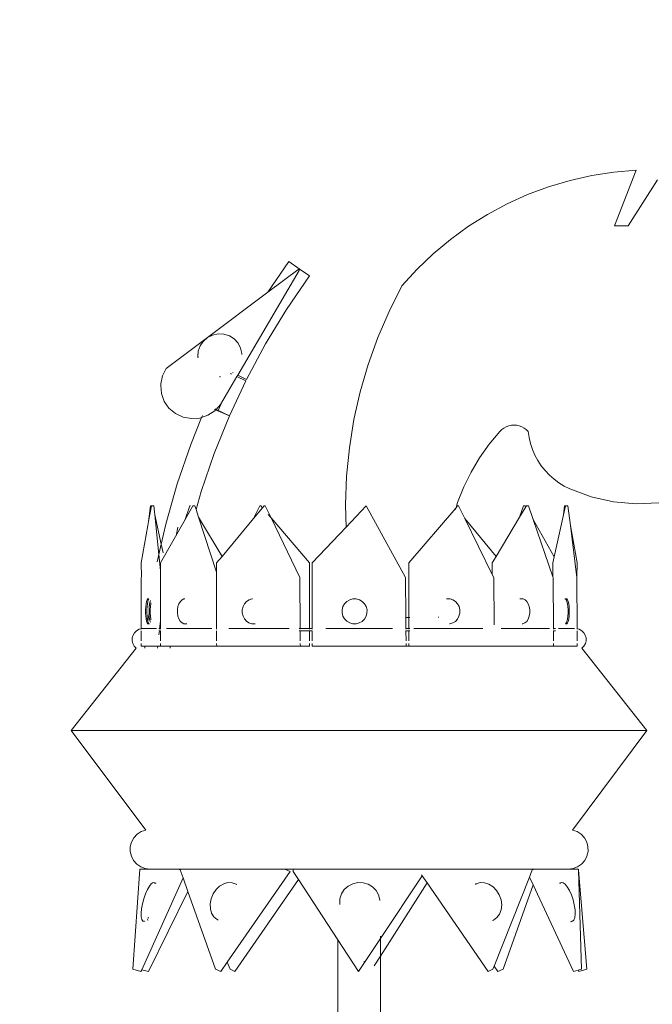
# Model space of a CAD drawing. Units: millimetres. Extents: x 7894 to 8038, y 6851 to 6951.
# Tile 33 of 49: x 7962.874 to 7964.635, y 6925.713 to 6928.453. Entities that reach past the tile are written whole.
import ezdxf

# ---------------------------------------------------------------- set-up
doc = ezdxf.new("R2010")
doc.units = ezdxf.units.MM
doc.layers.add('A-ANNO-DIMS', color=2, linetype='Continuous', lineweight=18)
doc.layers.add('A-FURN-ACCS', color=8, linetype='Continuous', lineweight=13)
doc.styles.get("Standard").update_dxf_attribs({"font": 'arial.ttf'})
doc.dimstyles.new('ISO-25', dxfattribs={"dimtxt": 1, "dimasz": 1, "dimexe": 1.25, "dimexo": 0.625, "dimtad": 1, "dimdec": 0, "dimlunit": 4, "dimtxsty": 'Standard', "dimcen": 2.5, "dimclrt": 1, "dimadec": 0, "dimazin": 0, "dimtfac": 1, "dimtdec": 0, "dimtmove": 0, "dimatfit": 3, "dimfxl": 1, "dimarcsym": 0})

# ---------------------------------------------------------------- blocks, each defined once
blk = doc.blocks.new('DISPLAY-LEAF-FINIAL-Z2_152')
for p, q in [((1.5102, 3.1734, 2.1518), (1.5723, 3.1787, 2.1518)), ((1.5723, 3.1787, 2.1518), (1.5113, 3.0242, 2.1518)), ((1.3879, 3.1503, 2.1518), (1.4486, 3.1639, 2.1518)), ((1.4486, 3.1639, 2.1518), (1.5102, 3.1734, 2.1518)), ((1.5498, 3.0242, 2.1518), (1.6318, 3.1522, 2.1518)), ((1.2698, 3.1109, 2.1518), (1.3281, 3.1326, 2.1518)), ((1.3281, 3.1326, 2.1518), (1.3879, 3.1503, 2.1518)), ((1.213, 3.0852, 2.1518), (1.2698, 3.1109, 2.1518)), ((1.1581, 3.0558, 2.1518), (1.213, 3.0852, 2.1518)), ((1.1053, 3.0227, 2.1518), (1.1581, 3.0558, 2.1518)), ((1.0549, 2.9861, 2.1518), (1.1053, 3.0227, 2.1518)), ((1.5113, 3.0242, 2.1518), (1.5498, 3.0242, 2.1518)), ((1.0071, 2.9462, 2.1518), (1.0549, 2.9861, 2.1518)), ((0.9621, 2.9031, 2.1518), (1.0071, 2.9462, 2.1518)), ((0.6052, 2.9244, 2.1518), (0.5471, 2.8395, 2.1518)), ((0.634, 2.9046, 2.1518), (0.5471, 2.8395, 2.1518)), ((0.634, 2.9046, 2.1518), (0.6052, 2.9244, 2.1518)), ((0.634, 2.9001, 2.1518), (0.634, 2.9046, 2.1518)), ((0.6629, 2.8848, 2.1518), (0.634, 2.9046, 2.1518)), ((0.634, 2.9001, 2.1518), (0.4632, 2.6089, 2.1518)), ((0.5989, 2.7915, 2.1518), (0.6629, 2.8848, 2.1518)), ((0.9202, 2.857, 2.1518), (0.9621, 2.9031, 2.1518)), ((0.9202, 2.857, 2.1518), (0.8844, 2.7861, 2.1518)), ((0.5471, 2.8395, 2.1518), (0.379, 2.7129, 2.1518)), ((0.5406, 2.6956, 2.1518), (0.5989, 2.7915, 2.1518)), ((0.8844, 2.7861, 2.1518), (0.8529, 2.7132, 2.1518)), ((0.379, 2.7129, 2.1518), (0.2637, 2.6275, 2.1518)), ((0.3671, 2.7026, 2.1518), (0.379, 2.7129, 2.1518)), ((0.379, 2.7129, 2.1518), (0.3932, 2.7199, 2.1518)), ((0.3932, 2.7199, 2.1518), (0.4088, 2.7231, 2.1518)), ((0.4088, 2.7231, 2.1518), (0.4248, 2.7223, 2.1518)), ((0.4248, 2.7223, 2.1518), (0.44, 2.7176, 2.1518)), ((0.44, 2.7176, 2.1518), (0.4533, 2.7092, 2.1518)), ((0.8529, 2.7132, 2.1518), (0.8261, 2.6384, 2.1518)), ((0.3535, 2.675, 2.1518), (0.3584, 2.6897, 2.1518)), ((0.3584, 2.6897, 2.1518), (0.3671, 2.7026, 2.1518)), ((0.4533, 2.7092, 2.1518), (0.464, 2.6977, 2.1518)), ((0.464, 2.6977, 2.1518), (0.4713, 2.6839, 2.1518)), ((0.5406, 2.6956, 2.1518), (0.4875, 2.5967, 2.1518)), ((0.3526, 2.6596, 2.1518), (0.3535, 2.675, 2.1518)), ((0.3527, 2.6591, 2.1518), (0.3526, 2.6596, 2.1518)), ((0.3526, 2.6569, 2.1518), (0.3527, 2.6591, 2.1518)), ((0.4713, 2.6839, 2.1518), (0.4746, 2.6689, 2.1518)), ((0.4745, 2.6667, 2.1518), (0.4746, 2.6689, 2.1518)), ((0.4745, 2.6667, 2.1518), (0.4746, 2.6661, 2.1518)), ((0.8261, 2.6384, 2.1518), (0.804, 2.5622, 2.1518)), ((0.2535, 2.6069, 2.1518), (0.249, 2.5845, 2.1518)), ((0.2637, 2.6275, 2.1518), (0.2535, 2.6069, 2.1518)), ((0.4144, 2.6055, 2.1518), (0.4132, 2.6029, 2.1518)), ((0.4608, 2.6047, 2.1518), (0.4152, 2.527, 2.1518)), ((0.4431, 2.613, 2.1518), (0.4459, 2.6117, 2.1518)), ((0.4508, 2.6151, 2.1518), (0.4489, 2.6161, 2.1518)), ((0.4632, 2.6089, 2.1518), (0.4608, 2.6047, 2.1518)), ((0.4858, 2.593, 2.1518), (0.4608, 2.6047, 2.1518)), ((0.4632, 2.6089, 2.1518), (0.4875, 2.5967, 2.1518)), ((0.249, 2.58, 2.1518), (0.249, 2.5845, 2.1518)), ((0.249, 2.58, 2.1518), (0.2508, 2.5572, 2.1518)), ((0.4402, 2.4957, 2.1518), (0.4858, 2.593, 2.1518)), ((0.2508, 2.5572, 2.1518), (0.2586, 2.5356, 2.1518)), ((0.804, 2.5622, 2.1518), (0.7865, 2.4847, 2.1518)), ((0.2586, 2.5356, 2.1518), (0.2719, 2.5167, 2.1518)), ((0.4029, 2.5132, 2.1518), (0.4152, 2.527, 2.1518)), ((0.4202, 2.5355, 2.1518), (0.4085, 2.5106, 2.1518)), ((0.2719, 2.5167, 2.1518), (0.2898, 2.5018, 2.1518)), ((0.2898, 2.5018, 2.1518), (0.3111, 2.4919, 2.1518)), ((0.3628, 2.4909, 2.1518), (0.3802, 2.4968, 2.1518)), ((0.3649, 2.4962, 2.1518), (0.3628, 2.4909, 2.1518)), ((0.3802, 2.4968, 2.1518), (0.3998, 2.5097, 2.1518)), ((0.3978, 2.391, 2.1518), (0.4399, 2.4951, 2.1518)), ((0.3983, 2.5132, 2.1518), (0.4016, 2.5117, 2.1518)), ((0.3998, 2.5097, 2.1518), (0.4016, 2.5117, 2.1518)), ((0.4029, 2.5132, 2.1518), (0.4003, 2.5144, 2.1518)), ((0.4016, 2.5117, 2.1518), (0.4029, 2.5132, 2.1518)), ((0.4016, 2.5117, 2.1518), (0.4399, 2.4951, 2.1518)), ((0.4029, 2.5132, 2.1518), (0.4402, 2.4957, 2.1518)), ((0.4085, 2.5106, 2.1518), (0.4078, 2.509, 2.1518)), ((0.3111, 2.4919, 2.1518), (0.3343, 2.4876, 2.1518)), ((0.3628, 2.4909, 2.1518), (0.3323, 2.4155, 2.1518)), ((0.3343, 2.4876, 2.1518), (0.3579, 2.4893, 2.1518)), ((0.3579, 2.4893, 2.1518), (0.3628, 2.4909, 2.1518)), ((0.7865, 2.4847, 2.1518), (0.774, 2.4062, 2.1518)), ((1.2175, 2.4675, 2.1518), (1.2106, 2.465, 2.1518)), ((1.2247, 2.469, 2.1518), (1.2175, 2.4675, 2.1518)), ((1.2321, 2.4695, 2.1518), (1.2247, 2.469, 2.1518)), ((1.2395, 2.469, 2.1518), (1.2321, 2.4695, 2.1518)), ((1.2467, 2.4675, 2.1518), (1.2395, 2.469, 2.1518)), ((1.2536, 2.465, 2.1518), (1.2467, 2.4675, 2.1518)), ((1.1928, 2.4521, 2.1518), (1.1631, 2.4165, 2.1518)), ((1.1981, 2.4572, 2.1518), (1.1928, 2.4521, 2.1518)), ((1.2041, 2.4615, 2.1518), (1.1981, 2.4572, 2.1518)), ((1.2106, 2.465, 2.1518), (1.2041, 2.4615, 2.1518)), ((1.2601, 2.4615, 2.1518), (1.2536, 2.465, 2.1518)), ((1.2661, 2.4572, 2.1518), (1.2601, 2.4615, 2.1518)), ((1.2714, 2.4521, 2.1518), (1.2661, 2.4572, 2.1518)), ((1.274, 2.435, 2.1518), (1.2714, 2.4521, 2.1518)), ((0.3323, 2.4155, 2.1518), (0.2946, 2.3057, 2.1518)), ((1.1631, 2.4165, 2.1518), (1.1364, 2.3788, 2.1518)), ((1.278, 2.4183, 2.1518), (1.274, 2.435, 2.1518)), ((1.2834, 2.4019, 2.1518), (1.278, 2.4183, 2.1518)), ((0.3614, 2.2848, 2.1518), (0.3978, 2.391, 2.1518)), ((0.774, 2.4062, 2.1518), (0.7662, 2.3272, 2.1518)), ((1.2903, 2.3861, 2.1518), (1.2834, 2.4019, 2.1518)), ((1.2985, 2.371, 2.1518), (1.2903, 2.3861, 2.1518)), ((1.1364, 2.3788, 2.1518), (1.1127, 2.339, 2.1518)), ((1.308, 2.3566, 2.1518), (1.2985, 2.371, 2.1518)), ((1.3187, 2.3431, 2.1518), (1.308, 2.3566, 2.1518)), ((1.1127, 2.339, 2.1518), (1.0923, 2.2975, 2.1518)), ((1.3305, 2.3306, 2.1518), (1.3187, 2.3431, 2.1518)), ((1.3434, 2.3192, 2.1518), (1.3305, 2.3306, 2.1518)), ((0.2946, 2.3057, 2.1518), (0.263, 2.1941, 2.1518)), ((0.7662, 2.3272, 2.1518), (0.7634, 2.2478, 2.1518)), ((1.3572, 2.3089, 2.1518), (1.3434, 2.3192, 2.1518)), ((1.3719, 2.2999, 2.1518), (1.3572, 2.3089, 2.1518)), ((0.3472, 2.2349, 2.1518), (0.3614, 2.2848, 2.1518)), ((1.0923, 2.2975, 2.1518), (1.0752, 2.2545, 2.1518)), ((1.3873, 2.2921, 2.1518), (1.3719, 2.2999, 2.1518)), ((1.4468, 2.2701, 2.1518), (1.3873, 2.2921, 2.1518)), ((0.7634, 2.2478, 2.1518), (0.7651, 2.1857, 2.1518)), ((1.0752, 2.2545, 2.1518), (1.0707, 2.2401, 2.1518)), ((1.5088, 2.256, 2.1518), (1.4468, 2.2701, 2.1518)), ((1.572, 2.2503, 2.1518), (1.5088, 2.256, 2.1518)), ((1.6354, 2.2529, 2.1518), (1.572, 2.2503, 2.1518)), ((0.2147, 2.201, 2.1518), (0.2202, 2.2445, 2.1518)), ((0.223, 2.2445, 2.1518), (0.2147, 2.201, 2.1518)), ((0.223, 2.2445, 2.1518), (0.2202, 2.2445, 2.1518)), ((0.223, 2.2445, 2.1518), (0.2299, 2.2445, 2.1518)), ((0.2325, 2.2195, 2.1518), (0.2299, 2.2445, 2.1518)), ((0.2325, 2.2195, 2.1518), (0.2504, 2.1381, 2.1518)), ((0.2439, 2.1095, 2.1518), (0.2325, 2.2195, 2.1518)), ((0.3171, 2.2068, 2.1518), (0.3302, 2.2445, 2.1518)), ((0.3384, 2.2445, 2.1518), (0.3171, 2.2068, 2.1518)), ((0.3318, 2.2445, 2.1518), (0.3302, 2.2445, 2.1518)), ((0.344, 2.2445, 2.1518), (0.3384, 2.2445, 2.1518)), ((0.3472, 2.2349, 2.1518), (0.344, 2.2445, 2.1518)), ((0.3543, 2.2133, 2.1518), (0.3472, 2.2349, 2.1518)), ((0.5072, 2.2093, 2.1518), (0.5246, 2.2445, 2.1518)), ((0.5322, 2.2392, 2.1518), (0.5072, 2.2093, 2.1518)), ((0.5277, 2.2445, 2.1518), (0.5246, 2.2445, 2.1518)), ((0.5277, 2.2445, 2.1518), (0.5322, 2.2392, 2.1518)), ((0.5366, 2.2445, 2.1518), (0.5322, 2.2392, 2.1518)), ((0.5399, 2.2445, 2.1518), (0.5366, 2.2445, 2.1518)), ((0.5559, 2.2114, 2.1518), (0.5399, 2.2445, 2.1518)), ((0.5482, 2.2204, 2.1518), (0.5559, 2.2114, 2.1518)), ((0.8207, 2.2445, 2.1518), (0.7651, 2.1857, 2.1518)), ((0.93, 2.0453, 2.1518), (0.8207, 2.2445, 2.1518)), ((1.0703, 2.2388, 2.1518), (0.9393, 2.0859, 2.1518)), ((1.0703, 2.2388, 2.1518), (1.069, 2.2345, 2.1518)), ((1.0707, 2.2401, 2.1518), (1.0703, 2.2388, 2.1518)), ((1.0703, 2.2388, 2.1518), (1.0715, 2.2374, 2.1518)), ((1.0745, 2.2445, 2.1518), (1.0707, 2.2401, 2.1518)), ((1.0745, 2.2445, 2.1518), (1.0775, 2.2445, 2.1518)), ((1.0949, 2.2093, 2.1518), (1.0775, 2.2445, 2.1518)), ((1.2478, 2.2133, 2.1518), (1.2581, 2.2445, 2.1518)), ((1.2651, 2.2421, 2.1518), (1.2478, 2.2133, 2.1518)), ((1.2581, 2.2445, 2.1518), (1.2637, 2.2445, 2.1518)), ((1.2637, 2.2445, 2.1518), (1.2651, 2.2421, 2.1518)), ((1.2666, 2.2445, 2.1518), (1.2651, 2.2421, 2.1518)), ((1.2666, 2.2445, 2.1518), (1.272, 2.2445, 2.1518)), ((1.2851, 2.2068, 2.1518), (1.272, 2.2445, 2.1518)), ((1.3696, 2.2195, 2.1518), (1.344, 2.1028, 2.1518)), ((1.3696, 2.2195, 2.1518), (1.3722, 2.2445, 2.1518)), ((1.3751, 2.2445, 2.1518), (1.3696, 2.2195, 2.1518)), ((1.3722, 2.2445, 2.1518), (1.3751, 2.2445, 2.1518)), ((1.3751, 2.2445, 2.1518), (1.3819, 2.2445, 2.1518)), ((1.3819, 2.2445, 2.1518), (1.3889, 2.1901, 2.1518)), ((0.2133, 2.1901, 2.1518), (0.2147, 2.201, 2.1518)), ((0.3171, 2.2068, 2.1518), (0.2485, 2.0859, 2.1518)), ((0.263, 2.1941, 2.1518), (0.2504, 2.1381, 2.1518)), ((0.3543, 2.2133, 2.1518), (0.4197, 2.1042, 2.1518)), ((0.4044, 2.0607, 2.1518), (0.3543, 2.2133, 2.1518)), ((0.5072, 2.2093, 2.1518), (0.4197, 2.1042, 2.1518)), ((0.5559, 2.2114, 2.1518), (0.6628, 2.0859, 2.1518)), ((0.636, 2.0453, 2.1518), (0.5559, 2.2114, 2.1518)), ((1.0949, 2.2093, 2.1518), (1.1824, 2.1042, 2.1518)), ((1.0949, 2.2093, 2.1518), (1.1714, 2.0542, 2.1518)), ((1.2478, 2.2133, 2.1518), (1.1824, 2.1042, 2.1518)), ((1.2851, 2.2068, 2.1518), (1.344, 2.1028, 2.1518)), ((1.2851, 2.2068, 2.1518), (1.3403, 2.0478, 2.1518)), ((0.2133, 2.1901, 2.1518), (0.1946, 2.0859, 2.1518)), ((0.2969, 2.1855, 2.1518), (0.2915, 2.1618, 2.1518)), ((0.7651, 2.1857, 2.1518), (0.6705, 2.0859, 2.1518)), ((1.3889, 2.1901, 2.1518), (1.4075, 2.0859, 2.1518)), ((1.4073, 2.0453, 2.1518), (1.3889, 2.1901, 2.1518)), ((0.2504, 2.1381, 2.1518), (0.2439, 2.1095, 2.1518)), ((0.2504, 2.1381, 2.1518), (0.2555, 2.1145, 2.1518)), ((0.1946, 2.0859, 2.1518), (0.1952, 2.0478, 2.1518)), ((0.2439, 2.1095, 2.1518), (0.2392, 2.0887, 2.1518)), ((0.2485, 2.0654, 2.1518), (0.2439, 2.1095, 2.1518)), ((0.2485, 2.0859, 2.1518), (0.2485, 2.0654, 2.1518)), ((0.4197, 2.1042, 2.1518), (0.4044, 2.0859, 2.1518)), ((0.4044, 2.0859, 2.1518), (0.4044, 2.0607, 2.1518)), ((0.6628, 2.0859, 2.1518), (0.6628, 1.9035, 2.1518)), ((0.6705, 2.0859, 2.1518), (0.6705, 1.9035, 2.1518)), ((0.9393, 2.0859, 2.1518), (0.9393, 1.9343, 2.1518)), ((1.1824, 2.1042, 2.1518), (1.1714, 2.0859, 2.1518)), ((1.1714, 2.0859, 2.1518), (1.1714, 2.0542, 2.1518)), ((1.344, 2.1028, 2.1518), (1.3403, 2.0859, 2.1518)), ((1.3403, 2.0859, 2.1518), (1.3403, 2.0478, 2.1518)), ((1.4075, 2.0859, 2.1518), (1.4073, 2.0453, 2.1518)), ((0.2485, 2.0654, 2.1518), (0.2485, 1.9035, 2.1518)), ((0.4044, 2.0607, 2.1518), (0.4044, 1.9015, 2.1518)), ((0.1949, 2.0453, 2.1518), (0.1946, 1.903, 2.1518)), ((0.1949, 2.0453, 2.1518), (0.1952, 2.0478, 2.1518)), ((0.636, 2.0453, 2.1518), (0.6371, 1.9035, 2.1518)), ((0.93, 2.0453, 2.1518), (0.9309, 1.9342, 2.1518)), ((1.1758, 2.0453, 2.1518), (1.1714, 2.0542, 2.1518)), ((1.1758, 2.0453, 2.1518), (1.1768, 1.9142, 2.1518)), ((1.3412, 2.0453, 2.1518), (1.3403, 2.0478, 2.1518)), ((1.3412, 2.0453, 2.1518), (1.3419, 1.9035, 2.1518)), ((1.4073, 2.0453, 2.1518), (1.4075, 1.903, 2.1518)), ((0.2074, 1.9648, 2.1518), (0.2082, 1.9727, 2.1518)), ((0.2082, 1.9727, 2.1518), (0.2095, 1.9791, 2.1518)), ((0.2095, 1.9791, 2.1518), (0.211, 1.9837, 2.1518)), ((0.2108, 1.9648, 2.1518), (0.2117, 1.9727, 2.1518)), ((0.211, 1.9837, 2.1518), (0.2126, 1.986, 2.1518)), ((0.2117, 1.9727, 2.1518), (0.2129, 1.9791, 2.1518)), ((0.2161, 1.986, 2.1518), (0.2126, 1.986, 2.1518)), ((0.2129, 1.9791, 2.1518), (0.2144, 1.9837, 2.1518)), ((0.2144, 1.9837, 2.1518), (0.2161, 1.986, 2.1518)), ((0.2194, 1.979, 2.1518), (0.2179, 1.9725, 2.1518)), ((0.2202, 1.9812, 2.1518), (0.2194, 1.979, 2.1518)), ((0.2204, 1.9806, 2.1518), (0.2194, 1.979, 2.1518)), ((0.2218, 1.9746, 2.1518), (0.2213, 1.9725, 2.1518)), ((0.2969, 1.9648, 2.1518), (0.2996, 1.9727, 2.1518)), ((0.2996, 1.9727, 2.1518), (0.3035, 1.9791, 2.1518)), ((0.3035, 1.9791, 2.1518), (0.3083, 1.9837, 2.1518)), ((0.3083, 1.9837, 2.1518), (0.3135, 1.986, 2.1518)), ((0.3163, 1.986, 2.1518), (0.3135, 1.986, 2.1518)), ((0.478, 1.9648, 2.1518), (0.482, 1.9727, 2.1518)), ((0.482, 1.9727, 2.1518), (0.4877, 1.9791, 2.1518)), ((0.4877, 1.9791, 2.1518), (0.4947, 1.9837, 2.1518)), ((0.4947, 1.9837, 2.1518), (0.5025, 1.986, 2.1518)), ((0.5041, 1.986, 2.1518), (0.5025, 1.986, 2.1518)), ((0.756, 1.9648, 2.1518), (0.7606, 1.9727, 2.1518)), ((0.7606, 1.9727, 2.1518), (0.7671, 1.9791, 2.1518)), ((0.7671, 1.9791, 2.1518), (0.775, 1.9837, 2.1518)), ((0.775, 1.9837, 2.1518), (0.7838, 1.986, 2.1518)), ((0.7838, 1.986, 2.1518), (0.7929, 1.986, 2.1518)), ((0.7929, 1.986, 2.1518), (0.8018, 1.9836, 2.1518)), ((0.8018, 1.9836, 2.1518), (0.8096, 1.979, 2.1518)), ((0.8096, 1.979, 2.1518), (0.8161, 1.9725, 2.1518)), ((1.0443, 1.986, 2.1518), (1.0459, 1.986, 2.1518)), ((1.0459, 1.986, 2.1518), (1.0541, 1.986, 2.1518)), ((1.0541, 1.986, 2.1518), (1.062, 1.9836, 2.1518)), ((1.062, 1.9836, 2.1518), (1.0691, 1.979, 2.1518)), ((1.0691, 1.979, 2.1518), (1.0749, 1.9725, 2.1518)), ((1.2486, 1.986, 2.1518), (1.2513, 1.986, 2.1518)), ((1.2513, 1.986, 2.1518), (1.2571, 1.986, 2.1518)), ((1.2571, 1.986, 2.1518), (1.2627, 1.9836, 2.1518)), ((1.2627, 1.9836, 2.1518), (1.2677, 1.979, 2.1518)), ((1.2677, 1.979, 2.1518), (1.2717, 1.9725, 2.1518)), ((1.3734, 1.986, 2.1518), (1.3755, 1.986, 2.1518)), ((1.3755, 1.986, 2.1518), (1.3775, 1.9836, 2.1518)), ((1.3755, 1.986, 2.1518), (1.3768, 1.986, 2.1518)), ((1.3768, 1.986, 2.1518), (1.3789, 1.986, 2.1518)), ((1.3775, 1.9836, 2.1518), (1.3794, 1.979, 2.1518)), ((1.3789, 1.986, 2.1518), (1.3809, 1.9836, 2.1518)), ((1.3794, 1.979, 2.1518), (1.3809, 1.9725, 2.1518)), ((1.3809, 1.9836, 2.1518), (1.3828, 1.979, 2.1518)), ((1.3828, 1.979, 2.1518), (1.3843, 1.9725, 2.1518)), ((0.2069, 1.956, 2.1518), (0.2074, 1.9648, 2.1518)), ((0.2069, 1.9469, 2.1518), (0.2069, 1.956, 2.1518)), ((0.2073, 1.938, 2.1518), (0.2069, 1.9469, 2.1518)), ((0.2103, 1.956, 2.1518), (0.2108, 1.9648, 2.1518)), ((0.2103, 1.9469, 2.1518), (0.2103, 1.956, 2.1518)), ((0.2108, 1.938, 2.1518), (0.2103, 1.9469, 2.1518)), ((0.2163, 1.9467, 2.1518), (0.2129, 1.9237, 2.1518)), ((0.2168, 1.9646, 2.1518), (0.2163, 1.9558, 2.1518)), ((0.2163, 1.9558, 2.1518), (0.2163, 1.9467, 2.1518)), ((0.2163, 1.9467, 2.1518), (0.2168, 1.9379, 2.1518)), ((0.2179, 1.9725, 2.1518), (0.2168, 1.9646, 2.1518)), ((0.218, 1.9665, 2.1518), (0.2168, 1.9646, 2.1518)), ((0.2179, 1.9725, 2.1518), (0.218, 1.9665, 2.1518)), ((0.2202, 1.9646, 2.1518), (0.2197, 1.9558, 2.1518)), ((0.2197, 1.9558, 2.1518), (0.2197, 1.9467, 2.1518)), ((0.2197, 1.9467, 2.1518), (0.2202, 1.9379, 2.1518)), ((0.2213, 1.9725, 2.1518), (0.2202, 1.9646, 2.1518)), ((0.2955, 1.956, 2.1518), (0.2969, 1.9648, 2.1518)), ((0.2955, 1.9469, 2.1518), (0.2955, 1.956, 2.1518)), ((0.2969, 1.938, 2.1518), (0.2955, 1.9469, 2.1518)), ((0.4759, 1.956, 2.1518), (0.478, 1.9648, 2.1518)), ((0.4759, 1.9469, 2.1518), (0.4759, 1.956, 2.1518)), ((0.4779, 1.938, 2.1518), (0.4759, 1.9469, 2.1518)), ((0.7536, 1.956, 2.1518), (0.756, 1.9648, 2.1518)), ((0.7536, 1.9469, 2.1518), (0.7536, 1.956, 2.1518)), ((0.756, 1.938, 2.1518), (0.7536, 1.9469, 2.1518)), ((0.8161, 1.9725, 2.1518), (0.8206, 1.9646, 2.1518)), ((0.8229, 1.9467, 2.1518), (0.8205, 1.9379, 2.1518)), ((0.8206, 1.9646, 2.1518), (0.823, 1.9558, 2.1518)), ((0.823, 1.9558, 2.1518), (0.8229, 1.9467, 2.1518)), ((1.0749, 1.9725, 2.1518), (1.079, 1.9646, 2.1518)), ((1.081, 1.9467, 2.1518), (1.0789, 1.9379, 2.1518)), ((1.079, 1.9646, 2.1518), (1.0811, 1.9558, 2.1518)), ((1.0811, 1.9558, 2.1518), (1.081, 1.9467, 2.1518)), ((1.2717, 1.9725, 2.1518), (1.2746, 1.9646, 2.1518)), ((1.2746, 1.9646, 2.1518), (1.2761, 1.9558, 2.1518)), ((1.2761, 1.9467, 2.1518), (1.2746, 1.9379, 2.1518)), ((1.2761, 1.9558, 2.1518), (1.2761, 1.9467, 2.1518)), ((1.3809, 1.9725, 2.1518), (1.3819, 1.9646, 2.1518)), ((1.3819, 1.9646, 2.1518), (1.3825, 1.9558, 2.1518)), ((1.3824, 1.9467, 2.1518), (1.3819, 1.9379, 2.1518)), ((1.3825, 1.9558, 2.1518), (1.3824, 1.9467, 2.1518)), ((1.3843, 1.9725, 2.1518), (1.3853, 1.9646, 2.1518)), ((1.3853, 1.9646, 2.1518), (1.3859, 1.9558, 2.1518)), ((1.3858, 1.9467, 2.1518), (1.3853, 1.9379, 2.1518)), ((1.3859, 1.9558, 2.1518), (1.3858, 1.9467, 2.1518)), ((0.2082, 1.9301, 2.1518), (0.2073, 1.938, 2.1518)), ((0.2094, 1.9237, 2.1518), (0.2082, 1.9301, 2.1518)), ((0.2109, 1.9191, 2.1518), (0.2094, 1.9237, 2.1518)), ((0.2116, 1.9301, 2.1518), (0.2108, 1.938, 2.1518)), ((0.2126, 1.9167, 2.1518), (0.2109, 1.9191, 2.1518)), ((0.2129, 1.9237, 2.1518), (0.2116, 1.9301, 2.1518)), ((0.2143, 1.9191, 2.1518), (0.2129, 1.9237, 2.1518)), ((0.216, 1.9167, 2.1518), (0.2143, 1.9191, 2.1518)), ((0.2168, 1.9379, 2.1518), (0.2179, 1.93, 2.1518)), ((0.2179, 1.93, 2.1518), (0.2194, 1.9235, 2.1518)), ((0.2194, 1.9235, 2.1518), (0.2202, 1.9215, 2.1518)), ((0.2202, 1.9379, 2.1518), (0.2213, 1.93, 2.1518)), ((0.2213, 1.93, 2.1518), (0.2218, 1.928, 2.1518)), ((0.2485, 1.9251, 2.1518), (0.2458, 1.9015, 2.1518)), ((0.2996, 1.9301, 2.1518), (0.2969, 1.938, 2.1518)), ((0.3034, 1.9237, 2.1518), (0.2996, 1.9301, 2.1518)), ((0.3082, 1.9191, 2.1518), (0.3034, 1.9237, 2.1518)), ((0.3134, 1.9167, 2.1518), (0.3082, 1.9191, 2.1518)), ((0.4819, 1.9301, 2.1518), (0.4779, 1.938, 2.1518)), ((0.4876, 1.9237, 2.1518), (0.4819, 1.9301, 2.1518)), ((0.4945, 1.9191, 2.1518), (0.4876, 1.9237, 2.1518)), ((0.5023, 1.9167, 2.1518), (0.4945, 1.9191, 2.1518)), ((0.7605, 1.9301, 2.1518), (0.756, 1.938, 2.1518)), ((0.7669, 1.9237, 2.1518), (0.7605, 1.9301, 2.1518)), ((0.7748, 1.9191, 2.1518), (0.7669, 1.9237, 2.1518)), ((0.7836, 1.9167, 2.1518), (0.7748, 1.9191, 2.1518)), ((0.8016, 1.919, 2.1518), (0.7928, 1.9167, 2.1518)), ((0.8095, 1.9235, 2.1518), (0.8016, 1.919, 2.1518)), ((0.816, 1.93, 2.1518), (0.8095, 1.9235, 2.1518)), ((0.8205, 1.9379, 2.1518), (0.816, 1.93, 2.1518)), ((0.9393, 1.9343, 2.1518), (0.9309, 1.9342, 2.1518)), ((0.9309, 1.9342, 2.1518), (0.9312, 1.9035, 2.1518)), ((0.9424, 1.9343, 2.1518), (0.9393, 1.9343, 2.1518)), ((0.9393, 1.9343, 2.1518), (0.9393, 1.9035, 2.1518)), ((1.0224, 1.935, 2.1518), (1.0208, 1.935, 2.1518)), ((1.0618, 1.919, 2.1518), (1.0539, 1.9167, 2.1518)), ((1.069, 1.9235, 2.1518), (1.0618, 1.919, 2.1518)), ((1.0748, 1.93, 2.1518), (1.069, 1.9235, 2.1518)), ((1.0789, 1.9379, 2.1518), (1.0748, 1.93, 2.1518)), ((1.2626, 1.919, 2.1518), (1.257, 1.9167, 2.1518)), ((1.2676, 1.9235, 2.1518), (1.2626, 1.919, 2.1518)), ((1.2717, 1.93, 2.1518), (1.2676, 1.9235, 2.1518)), ((1.2746, 1.9379, 2.1518), (1.2717, 1.93, 2.1518)), ((1.3775, 1.919, 2.1518), (1.3755, 1.9167, 2.1518)), ((1.3793, 1.9235, 2.1518), (1.3775, 1.919, 2.1518)), ((1.3809, 1.919, 2.1518), (1.3789, 1.9167, 2.1518)), ((1.3808, 1.93, 2.1518), (1.3793, 1.9235, 2.1518)), ((1.3819, 1.9379, 2.1518), (1.3808, 1.93, 2.1518)), ((1.3827, 1.9235, 2.1518), (1.3809, 1.919, 2.1518)), ((1.3842, 1.93, 2.1518), (1.3827, 1.9235, 2.1518)), ((1.3853, 1.9379, 2.1518), (1.3842, 1.93, 2.1518)), ((0.1719, 1.8852, 2.1518), (0.1759, 1.892, 2.1518)), ((0.1759, 1.892, 2.1518), (0.1817, 1.8976, 2.1518)), ((0.1817, 1.8976, 2.1518), (0.1886, 1.9015, 2.1518)), ((0.1886, 1.9015, 2.1518), (0.1946, 1.903, 2.1518)), ((0.1946, 1.8976, 2.1518), (0.1945, 1.8695, 2.1518)), ((0.1946, 1.903, 2.1518), (0.1964, 1.9035, 2.1518)), ((0.1946, 1.903, 2.1518), (0.1946, 1.9015, 2.1518)), ((0.1964, 1.9035, 2.1518), (0.1977, 1.9034, 2.1518)), ((0.1964, 1.9035, 2.1518), (0.1969, 1.9035, 2.1518)), ((0.2373, 1.9035, 2.1518), (0.1977, 1.9034, 2.1518)), ((0.2143, 1.9167, 2.1518), (0.2126, 1.9167, 2.1518)), ((0.216, 1.9167, 2.1518), (0.2143, 1.9167, 2.1518)), ((0.2177, 1.9167, 2.1518), (0.216, 1.9167, 2.1518)), ((0.2485, 1.9035, 2.1518), (0.2439, 1.9035, 2.1518)), ((0.2453, 1.8976, 2.1518), (0.2439, 1.8856, 2.1518)), ((0.2485, 1.8971, 2.1518), (0.2439, 1.8971, 2.1518)), ((0.2485, 1.9035, 2.1518), (0.2485, 1.9015, 2.1518)), ((0.2485, 1.8976, 2.1518), (0.2485, 1.8971, 2.1518)), ((0.2485, 1.8971, 2.1518), (0.2485, 1.8695, 2.1518)), ((0.3912, 1.9035, 2.1518), (0.265, 1.9035, 2.1518)), ((0.3189, 1.9167, 2.1518), (0.3134, 1.9167, 2.1518)), ((0.3217, 1.9167, 2.1518), (0.3189, 1.9167, 2.1518)), ((0.4044, 1.8976, 2.1518), (0.4044, 1.8695, 2.1518)), ((0.4385, 1.9035, 2.1518), (0.6066, 1.9035, 2.1518)), ((0.5103, 1.9167, 2.1518), (0.5023, 1.9167, 2.1518)), ((0.512, 1.9167, 2.1518), (0.5103, 1.9167, 2.1518)), ((0.6371, 1.9035, 2.1518), (0.6338, 1.9035, 2.1518)), ((0.6371, 1.8971, 2.1518), (0.6338, 1.8971, 2.1518)), ((0.6371, 1.9035, 2.1518), (0.6371, 1.9015, 2.1518)), ((0.6628, 1.9035, 2.1518), (0.6371, 1.9035, 2.1518)), ((0.6371, 1.8976, 2.1518), (0.6371, 1.8971, 2.1518)), ((0.6371, 1.8971, 2.1518), (0.6373, 1.8695, 2.1518)), ((0.6628, 1.8971, 2.1518), (0.6371, 1.8971, 2.1518)), ((0.6628, 1.9035, 2.1518), (0.6705, 1.9035, 2.1518)), ((0.6628, 1.9035, 2.1518), (0.6628, 1.9015, 2.1518)), ((0.6628, 1.8976, 2.1518), (0.6628, 1.8971, 2.1518)), ((0.6628, 1.8971, 2.1518), (0.6628, 1.8695, 2.1518)), ((0.6705, 1.8971, 2.1518), (0.6628, 1.8971, 2.1518)), ((0.6705, 1.9035, 2.1518), (0.6705, 1.9015, 2.1518)), ((0.6705, 1.8976, 2.1518), (0.6705, 1.8971, 2.1518)), ((0.6705, 1.8971, 2.1518), (0.6705, 1.8695, 2.1518)), ((0.7081, 1.9035, 2.1518), (0.894, 1.9035, 2.1518)), ((0.7928, 1.9167, 2.1518), (0.7836, 1.9167, 2.1518)), ((0.9312, 1.9035, 2.1518), (0.9312, 1.9015, 2.1518)), ((0.9393, 1.9035, 2.1518), (0.9312, 1.9035, 2.1518)), ((0.9313, 1.8976, 2.1518), (0.9313, 1.8971, 2.1518)), ((0.9313, 1.8971, 2.1518), (0.9315, 1.8695, 2.1518)), ((0.9393, 1.8971, 2.1518), (0.9313, 1.8971, 2.1518)), ((0.9424, 1.9035, 2.1518), (0.9393, 1.9035, 2.1518)), ((0.9393, 1.9035, 2.1518), (0.9393, 1.9015, 2.1518)), ((0.9393, 1.8976, 2.1518), (0.9393, 1.8971, 2.1518)), ((0.9424, 1.8971, 2.1518), (0.9393, 1.8971, 2.1518)), ((0.9393, 1.8971, 2.1518), (0.9393, 1.8695, 2.1518)), ((0.9534, 1.9035, 2.1518), (1.1456, 1.9035, 2.1518)), ((1.0524, 1.9167, 2.1518), (1.0539, 1.9167, 2.1518)), ((1.3304, 1.9035, 2.1518), (1.1965, 1.9035, 2.1518)), ((1.2543, 1.9167, 2.1518), (1.257, 1.9167, 2.1518)), ((1.3471, 1.9035, 2.1518), (1.3419, 1.9035, 2.1518)), ((1.3419, 1.9035, 2.1518), (1.342, 1.9015, 2.1518)), ((1.342, 1.8976, 2.1518), (1.342, 1.8971, 2.1518)), ((1.3471, 1.8971, 2.1518), (1.342, 1.8971, 2.1518)), ((1.342, 1.8971, 2.1518), (1.3421, 1.8695, 2.1518)), ((1.3561, 1.9035, 2.1518), (1.4004, 1.9035, 2.1518)), ((1.3755, 1.9167, 2.1518), (1.3789, 1.9167, 2.1518)), ((1.4075, 1.903, 2.1518), (1.4135, 1.9015, 2.1518)), ((1.4075, 1.903, 2.1518), (1.4075, 1.9015, 2.1518)), ((1.4075, 1.8976, 2.1518), (1.4075, 1.8695, 2.1518)), ((1.4135, 1.9015, 2.1518), (1.4205, 1.8976, 2.1518)), ((1.4205, 1.8976, 2.1518), (1.4262, 1.892, 2.1518)), ((1.4262, 1.892, 2.1518), (1.4303, 1.8852, 2.1518)), ((0.1696, 1.8695, 2.1518), (0.1697, 1.8775, 2.1518)), ((0.1715, 1.8618, 2.1518), (0.1696, 1.8695, 2.1518)), ((0.1697, 1.8775, 2.1518), (0.1719, 1.8852, 2.1518)), ((1.4303, 1.8852, 2.1518), (1.4325, 1.8775, 2.1518)), ((1.4326, 1.8695, 2.1518), (1.4306, 1.8618, 2.1518)), ((1.4325, 1.8775, 2.1518), (1.4326, 1.8695, 2.1518)), ((0, 1.6201, 2.1518), (0.181, 1.8491, 2.1518)), ((0.1754, 1.8548, 2.1518), (0.1715, 1.8618, 2.1518)), ((0.181, 1.8491, 2.1518), (0.1754, 1.8548, 2.1518)), ((0.1945, 1.8618, 2.1518), (0.1945, 1.8548, 2.1518)), ((0.1952, 1.8548, 2.1518), (0.1945, 1.8548, 2.1518)), ((0.2052, 1.8548, 2.1518), (0.1945, 1.8548, 2.1518)), ((0.2048, 1.8513, 2.1518), (0.2047, 1.8491, 2.1518)), ((0.2052, 1.8548, 2.1518), (0.2048, 1.8513, 2.1518)), ((0.2485, 1.8548, 2.1518), (0.2052, 1.8548, 2.1518)), ((0.2404, 1.8548, 2.1518), (0.2398, 1.8491, 2.1518)), ((0.2485, 1.8618, 2.1518), (0.2485, 1.8548, 2.1518)), ((0.2485, 1.8548, 2.1518), (0.2756, 1.8548, 2.1518)), ((0.2749, 1.8491, 2.1518), (0.2756, 1.8548, 2.1518)), ((0.2756, 1.8548, 2.1518), (0.4049, 1.8548, 2.1518)), ((0.4044, 1.8618, 2.1518), (0.4049, 1.8548, 2.1518)), ((0.4049, 1.8548, 2.1518), (0.6375, 1.8548, 2.1518)), ((0.6374, 1.8618, 2.1518), (0.6375, 1.8548, 2.1518)), ((0.6628, 1.8548, 2.1518), (0.6375, 1.8548, 2.1518)), ((0.6628, 1.8618, 2.1518), (0.6628, 1.8548, 2.1518)), ((0.6705, 1.8618, 2.1518), (0.6705, 1.8548, 2.1518)), ((0.6705, 1.8548, 2.1518), (0.9316, 1.8548, 2.1518)), ((0.9316, 1.8618, 2.1518), (0.9316, 1.8548, 2.1518)), ((0.9393, 1.8548, 2.1518), (0.9316, 1.8548, 2.1518)), ((0.9393, 1.8618, 2.1518), (0.9393, 1.8548, 2.1518)), ((1.3422, 1.8548, 2.1518), (0.9393, 1.8548, 2.1518)), ((1.3422, 1.8618, 2.1518), (1.3422, 1.8548, 2.1518)), ((1.4075, 1.8548, 2.1518), (1.3422, 1.8548, 2.1518)), ((1.4075, 1.8618, 2.1518), (1.4075, 1.8548, 2.1518)), ((1.4267, 1.8548, 2.1518), (1.4212, 1.8491, 2.1518)), ((1.4212, 1.8491, 2.1518), (1.6021, 1.6201, 2.1518)), ((1.4306, 1.8618, 2.1518), (1.4267, 1.8548, 2.1518)), ((0.2072, 1.3429, 2.1518), (0, 1.6201, 2.1518)), ((1.6021, 1.6201, 2.1518), (0, 1.6201, 2.1518)), ((1.6021, 1.6201, 2.1518), (1.395, 1.3429, 2.1518)), ((0.1945, 1.3385, 2.1518), (0.2072, 1.3429, 2.1518)), ((1.395, 1.3429, 2.1518), (1.4076, 1.3385, 2.1518)), ((0.1678, 1.3095, 2.1518), (0.1742, 1.3213, 2.1518)), ((0.1742, 1.3213, 2.1518), (0.1833, 1.3311, 2.1518)), ((0.1833, 1.3311, 2.1518), (0.1945, 1.3385, 2.1518)), ((1.4076, 1.3385, 2.1518), (1.4188, 1.3311, 2.1518)), ((1.4188, 1.3311, 2.1518), (1.4279, 1.3213, 2.1518)), ((1.4279, 1.3213, 2.1518), (1.4344, 1.3095, 2.1518)), ((0.1641, 1.2832, 2.1518), (0.1643, 1.2966, 2.1518)), ((0.1643, 1.2966, 2.1518), (0.1678, 1.3095, 2.1518)), ((1.4344, 1.3095, 2.1518), (1.4378, 1.2966, 2.1518)), ((1.4378, 1.2966, 2.1518), (1.438, 1.2832, 2.1518)), ((0.1672, 1.2701, 2.1518), (0.1641, 1.2832, 2.1518)), ((0.1733, 1.2582, 2.1518), (0.1672, 1.2701, 2.1518)), ((1.435, 1.2701, 2.1518), (1.4288, 1.2582, 2.1518)), ((1.438, 1.2832, 2.1518), (1.435, 1.2701, 2.1518)), ((0.1714, 0.9553, 2.1518), (0.1907, 1.234, 2.1518)), ((0.1821, 1.2481, 2.1518), (0.1733, 1.2582, 2.1518)), ((0.1931, 1.2404, 2.1518), (0.1821, 1.2481, 2.1518)), ((0.2189, 1.234, 2.1518), (0.1907, 1.234, 2.1518)), ((0.2056, 1.2356, 2.1518), (0.1931, 1.2404, 2.1518)), ((0.2189, 1.234, 2.1518), (0.2056, 1.2356, 2.1518)), ((0.2189, 1.234, 2.1518), (0.2969, 1.234, 2.1518)), ((0.2969, 1.234, 2.1518), (0.3022, 1.234, 2.1518)), ((0.3029, 1.2321, 2.1518), (0.2969, 1.234, 2.1518)), ((0.3029, 1.2321, 2.1518), (0.3022, 1.234, 2.1518)), ((0.3022, 1.234, 2.1518), (0.5943, 1.234, 2.1518)), ((0.5943, 1.234, 2.1518), (0.6175, 1.234, 2.1518)), ((0.6087, 1.2276, 2.1518), (0.5943, 1.234, 2.1518)), ((0.6175, 1.2276, 2.1518), (0.6175, 1.234, 2.1518)), ((0.9517, 1.234, 2.1518), (0.6175, 1.234, 2.1518)), ((0.9809, 1.2337, 2.1518), (0.9517, 1.234, 2.1518)), ((0.9809, 1.2337, 2.1518), (0.9815, 1.234, 2.1518)), ((0.9815, 1.234, 2.1518), (0.9829, 1.234, 2.1518)), ((1.2836, 1.234, 2.1518), (0.9829, 1.234, 2.1518)), ((1.2826, 1.2319, 2.1518), (1.2898, 1.234, 2.1518)), ((1.2826, 1.2319, 2.1518), (1.2836, 1.234, 2.1518)), ((1.2836, 1.234, 2.1518), (1.2898, 1.234, 2.1518)), ((1.2898, 1.234, 2.1518), (1.3832, 1.234, 2.1518)), ((1.3965, 1.2356, 2.1518), (1.3832, 1.234, 2.1518)), ((1.41, 1.2337, 2.1518), (1.3832, 1.234, 2.1518)), ((1.409, 1.2404, 2.1518), (1.3965, 1.2356, 2.1518)), ((1.42, 1.2481, 2.1518), (1.409, 1.2404, 2.1518)), ((1.4111, 1.234, 2.1518), (1.41, 1.2337, 2.1518)), ((1.4113, 1.2316, 2.1518), (1.4111, 1.234, 2.1518)), ((1.4288, 1.2582, 2.1518), (1.42, 1.2481, 2.1518)), ((0.1964, 0.9543, 2.1518), (0.3109, 1.2098, 2.1518)), ((0.3109, 1.2098, 2.1518), (0.3029, 1.2321, 2.1518)), ((0.3244, 1.1717, 2.1518), (0.3109, 1.2098, 2.1518)), ((0.4339, 0.9752, 2.1518), (0.6087, 1.2276, 2.1518)), ((0.6322, 1.205, 2.1518), (0.6175, 1.2276, 2.1518)), ((0.8605, 1.0411, 2.1518), (0.9765, 1.2154, 2.1518)), ((0.9765, 1.2154, 2.1518), (0.9744, 1.2185, 2.1518)), ((0.9902, 1.1955, 2.1518), (0.9765, 1.2154, 2.1518)), ((1.1768, 0.964, 2.1518), (1.2748, 1.2121, 2.1518)), ((1.2748, 1.2121, 2.1518), (1.2826, 1.2319, 2.1518)), ((1.285, 1.1903, 2.1518), (1.2748, 1.2121, 2.1518)), ((1.4348, 0.9553, 2.1518), (1.4113, 1.2316, 2.1518)), ((1.4203, 0.9553, 2.1518), (1.4113, 1.2316, 2.1518)), ((0.2118, 1.177, 2.1518), (0.2173, 1.1867, 2.1518)), ((0.2173, 1.1867, 2.1518), (0.2227, 1.1934, 2.1518)), ((0.2227, 1.1934, 2.1518), (0.2276, 1.1967, 2.1518)), ((0.2276, 1.1967, 2.1518), (0.2317, 1.1963, 2.1518)), ((0.2325, 1.1953, 2.1518), (0.2317, 1.1963, 2.1518)), ((0.2325, 1.1953, 2.1518), (0.2366, 1.1949, 2.1518)), ((0.4028, 1.177, 2.1518), (0.4128, 1.1867, 2.1518)), ((0.4128, 1.1867, 2.1518), (0.4241, 1.1934, 2.1518)), ((0.4241, 1.1934, 2.1518), (0.436, 1.1967, 2.1518)), ((0.436, 1.1967, 2.1518), (0.4475, 1.1963, 2.1518)), ((0.4475, 1.1963, 2.1518), (0.4584, 1.192, 2.1518)), ((0.455, 0.949, 2.1518), (0.6322, 1.205, 2.1518)), ((0.4584, 1.192, 2.1518), (0.4611, 1.1909, 2.1518)), ((0.7416, 1.0372, 2.1518), (0.6322, 1.205, 2.1518)), ((0.7597, 1.177, 2.1518), (0.7703, 1.1867, 2.1518)), ((0.7703, 1.1867, 2.1518), (0.7831, 1.1934, 2.1518)), ((0.7831, 1.1934, 2.1518), (0.7973, 1.1967, 2.1518)), ((0.7973, 1.1967, 2.1518), (0.8119, 1.1963, 2.1518)), ((0.8119, 1.1963, 2.1518), (0.8259, 1.1923, 2.1518)), ((0.8259, 1.1923, 2.1518), (0.8383, 1.1849, 2.1518)), ((0.8383, 1.1849, 2.1518), (0.8484, 1.1746, 2.1518)), ((0.8605, 0.9923, 2.1518), (0.9902, 1.1955, 2.1518)), ((1.1599, 0.949, 2.1518), (0.9902, 1.1955, 2.1518)), ((1.1241, 1.1921, 2.1518), (1.1257, 1.1926, 2.1518)), ((1.1257, 1.1926, 2.1518), (1.127, 1.1934, 2.1518)), ((1.127, 1.1934, 2.1518), (1.1382, 1.1967, 2.1518)), ((1.1382, 1.1967, 2.1518), (1.1502, 1.1963, 2.1518)), ((1.1502, 1.1963, 2.1518), (1.1623, 1.1923, 2.1518)), ((1.1623, 1.1923, 2.1518), (1.1737, 1.1849, 2.1518)), ((1.1737, 1.1849, 2.1518), (1.1835, 1.1746, 2.1518)), ((1.2015, 0.9553, 2.1518), (1.285, 1.1903, 2.1518)), ((1.398, 0.949, 2.1518), (1.285, 1.1903, 2.1518)), ((1.359, 1.1953, 2.1518), (1.3638, 1.1967, 2.1518)), ((1.359, 1.1953, 2.1518), (1.3619, 1.1951, 2.1518)), ((1.3638, 1.1967, 2.1518), (1.3687, 1.1963, 2.1518)), ((1.3687, 1.1963, 2.1518), (1.3744, 1.1923, 2.1518)), ((1.3744, 1.1923, 2.1518), (1.3804, 1.1849, 2.1518)), ((1.3804, 1.1849, 2.1518), (1.3863, 1.1746, 2.1518)), ((0.1981, 1.1374, 2.1518), (0.2018, 1.1515, 2.1518)), ((0.2018, 1.1515, 2.1518), (0.2065, 1.165, 2.1518)), ((0.2065, 1.165, 2.1518), (0.2118, 1.177, 2.1518)), ((0.2147, 0.949, 2.1518), (0.3244, 1.1717, 2.1518)), ((0.4015, 0.9553, 2.1518), (0.3244, 1.1717, 2.1518)), ((0.3867, 1.1374, 2.1518), (0.3893, 1.1515, 2.1518)), ((0.3893, 1.1515, 2.1518), (0.3948, 1.165, 2.1518)), ((0.3948, 1.165, 2.1518), (0.4028, 1.177, 2.1518)), ((0.7475, 1.1373, 2.1518), (0.7478, 1.1515, 2.1518)), ((0.7478, 1.1515, 2.1518), (0.752, 1.165, 2.1518)), ((0.752, 1.165, 2.1518), (0.7597, 1.177, 2.1518)), ((0.8484, 1.1746, 2.1518), (0.8553, 1.1622, 2.1518)), ((0.8553, 1.1622, 2.1518), (0.8587, 1.1485, 2.1518)), ((1.1835, 1.1746, 2.1518), (1.1911, 1.1622, 2.1518)), ((1.1911, 1.1622, 2.1518), (1.196, 1.1485, 2.1518)), ((1.3863, 1.1746, 2.1518), (1.3917, 1.1622, 2.1518)), ((1.3917, 1.1622, 2.1518), (1.3963, 1.1485, 2.1518)), ((0.1943, 1.1113, 2.1518), (0.1955, 1.1237, 2.1518)), ((0.1955, 1.1237, 2.1518), (0.1981, 1.1374, 2.1518)), ((0.3871, 1.1237, 2.1518), (0.3867, 1.1374, 2.1518)), ((0.3906, 1.1113, 2.1518), (0.3871, 1.1237, 2.1518)), ((0.7474, 1.1361, 2.1518), (0.7475, 1.1373, 2.1518)), ((0.8587, 1.1471, 2.1518), (0.8587, 1.1485, 2.1518)), ((1.196, 1.1485, 2.1518), (1.1978, 1.1344, 2.1518)), ((1.1978, 1.1344, 2.1518), (1.1964, 1.1209, 2.1518)), ((1.3963, 1.1485, 2.1518), (1.3997, 1.1344, 2.1518)), ((1.3997, 1.1344, 2.1518), (1.4018, 1.1209, 2.1518)), ((0.1946, 1.101, 2.1518), (0.1943, 1.1113, 2.1518)), ((0.1963, 1.0936, 2.1518), (0.1946, 1.101, 2.1518)), ((0.2112, 1.0961, 2.1518), (0.2129, 1.0925, 2.1518)), ((0.2141, 1.1, 2.1518), (0.2145, 1.0978, 2.1518)), ((0.3969, 1.101, 2.1518), (0.3906, 1.1113, 2.1518)), ((0.4056, 1.0936, 2.1518), (0.3969, 1.101, 2.1518)), ((1.1847, 1.0992, 2.1518), (1.1752, 1.0925, 2.1518)), ((1.192, 1.1089, 2.1518), (1.1847, 1.0992, 2.1518)), ((1.1964, 1.1209, 2.1518), (1.192, 1.1089, 2.1518)), ((1.4012, 1.0992, 2.1518), (1.3987, 1.0925, 2.1518)), ((1.4023, 1.1089, 2.1518), (1.4012, 1.0992, 2.1518)), ((1.4018, 1.1209, 2.1518), (1.4023, 1.1089, 2.1518)), ((0.1992, 1.0896, 2.1518), (0.1963, 1.0936, 2.1518)), ((0.2034, 1.0892, 2.1518), (0.1992, 1.0896, 2.1518)), ((0.2041, 1.0883, 2.1518), (0.2034, 1.0892, 2.1518)), ((0.2129, 1.0925, 2.1518), (0.2137, 1.0919, 2.1518)), ((0.4087, 1.0923, 2.1518), (0.4056, 1.0936, 2.1518)), ((1.1736, 1.092, 2.1518), (1.1723, 1.0911, 2.1518)), ((1.1736, 1.092, 2.1518), (1.1752, 1.0925, 2.1518)), ((1.3919, 1.0895, 2.1518), (1.39, 1.0879, 2.1518)), ((1.39, 1.0879, 2.1518), (1.3948, 1.0892, 2.1518)), ((1.3987, 1.0925, 2.1518), (1.3948, 1.0892, 2.1518)), ((0.8158, 0.974, 2.1518), (0.8605, 1.0411, 2.1518)), ((0.8605, 1.0411, 2.1518), (0.8605, 1.0475, 2.1518)), ((0.8605, 0.9923, 2.1518), (0.8605, 1.0411, 2.1518)), ((0.7416, 0, 2.1518), (0.7416, 1.0372, 2.1518)), ((0.7992, 0.949, 2.1518), (0.7416, 1.0372, 2.1518)), ((0.8431, 0.9651, 2.1518), (0.8605, 0.9923, 2.1518)), ((0.8605, 0, 2.1518), (0.8605, 0.9923, 2.1518)), ((0.4158, 0.949, 2.1518), (0.4339, 0.9752, 2.1518)), ((0.4421, 0.9553, 2.1518), (0.4339, 0.9752, 2.1518)), ((0.7992, 0.949, 2.1518), (0.8158, 0.974, 2.1518)), ((0.8158, 0.974, 2.1518), (0.8137, 0.9772, 2.1518)), ((0.8164, 0.9731, 2.1518), (0.8158, 0.974, 2.1518)), ((1.1734, 0.9553, 2.1518), (1.1768, 0.964, 2.1518)), ((1.1872, 0.949, 2.1518), (1.1768, 0.964, 2.1518)), ((0.194, 0.949, 2.1518), (0.1714, 0.9553, 2.1518)), ((0.194, 0.949, 2.1518), (0.1964, 0.9543, 2.1518)), ((0.2147, 0.949, 2.1518), (0.1964, 0.9543, 2.1518)), ((0.4158, 0.949, 2.1518), (0.4015, 0.9553, 2.1518)), ((0.455, 0.949, 2.1518), (0.4421, 0.9553, 2.1518)), ((1.1599, 0.949, 2.1518), (1.1734, 0.9553, 2.1518)), ((1.1872, 0.949, 2.1518), (1.2015, 0.9553, 2.1518)), ((1.398, 0.949, 2.1518), (1.4105, 0.9525, 2.1518)), ((1.4105, 0.9525, 2.1518), (1.4203, 0.9553, 2.1518)), ((1.412, 0.949, 2.1518), (1.4105, 0.9525, 2.1518)), ((1.412, 0.949, 2.1518), (1.4348, 0.9553, 2.1518))]:
    blk.add_line(p, q)
blk = doc.blocks.new('*D23')
at = {"layer": 'A-ANNO-DIMS', "color": 0, "lineweight": -2, "transparency": 16777216}
for p, q in [((7940.0888, 6907.098), (7940.0888, 6947.7928)), ((7971.9356, 6928.989), (7971.9356, 6947.7928)), ((7941.0888, 6946.5428), (7970.9356, 6946.5428))]:
    blk.add_line(p, q, dxfattribs=at)
at = {"layer": 'A-ANNO-DIMS', "color": 0, "transparency": 16777216}
for points in [[(7941.0888, 6946.7095), (7941.0888, 6946.3762), (7940.0888, 6946.5428)], [(7970.9356, 6946.7095), (7970.9356, 6946.3762), (7971.9356, 6946.5428)]]:
    blk.add_solid(points, dxfattribs=at)
at = {"layer": 'Defpoints', "color": 0, "transparency": 16777216}
for p in [(7971.9356, 6946.5428), (7971.9356, 6928.364), (7940.0888, 6906.473)]:
    blk.add_point(p, dxfattribs=at)
at = {"layer": 'A-ANNO-DIMS', "color": 1, "transparency": 16777216, "insert": (7956.0122, 6947.6784), "char_height": 1, "attachment_point": 5}
blk.add_mtext('2\'-8"', dxfattribs=at)
blk = doc.blocks.new('*D28')
at = {"layer": 'A-ANNO-DIMS', "color": 0, "lineweight": -2, "transparency": 16777216}
for p, q in [((7960.8854, 6936.8804), (7975.2272, 6936.8804)), ((7973.9772, 6935.8804), (7973.9772, 6923.6283)), ((7971.8421, 6922.6283), (7975.2272, 6922.6283))]:
    blk.add_line(p, q, dxfattribs=at)
at = {"layer": 'A-ANNO-DIMS', "color": 0, "transparency": 16777216}
for points in [[(7973.8105, 6935.8804), (7974.1439, 6935.8804), (7973.9772, 6936.8804)], [(7973.8105, 6923.6283), (7974.1439, 6923.6283), (7973.9772, 6922.6283)]]:
    blk.add_solid(points, dxfattribs=at)
at = {"layer": 'Defpoints', "color": 0, "transparency": 16777216}
for p in [(7960.2604, 6936.8804), (7971.2171, 6922.6283), (7973.9772, 6922.6283)]:
    blk.add_point(p, dxfattribs=at)
at = {"layer": 'A-ANNO-DIMS', "color": 1, "transparency": 16777216, "insert": (7972.8351, 6929.7543), "char_height": 1, "attachment_point": 5, "rotation": 90}
blk.add_mtext('1\'-2 1/2"', dxfattribs=at)
blk = doc.blocks.new('*D31')
at = {"layer": 'A-ANNO-DIMS', "color": 0, "lineweight": -2, "transparency": 16777216}
for p, q in [((7973.9772, 6921.7198), (7973.9772, 6926.628)), ((7949.8107, 6920.7198), (7975.2272, 6920.7198)), ((7973.9772, 6918.7198), (7973.9772, 6920.7198)), ((7950.9654, 6918.7198), (7975.2272, 6918.7198)), ((7973.9772, 6917.7198), (7973.9772, 6916.7198))]:
    blk.add_line(p, q, dxfattribs=at)
at = {"layer": 'A-ANNO-DIMS', "color": 0, "transparency": 16777216}
for points in [[(7973.8105, 6921.7198), (7974.1439, 6921.7198), (7973.9772, 6920.7198)], [(7973.8105, 6917.7198), (7974.1439, 6917.7198), (7973.9772, 6918.7198)]]:
    blk.add_solid(points, dxfattribs=at)
at = {"layer": 'Defpoints', "color": 0, "transparency": 16777216}
for p in [(7949.1857, 6920.7198), (7973.9772, 6920.7198), (7950.3404, 6918.7198)]:
    blk.add_point(p, dxfattribs=at)
at = {"layer": 'A-ANNO-DIMS', "color": 1, "transparency": 16777216, "insert": (7972.8416, 6924.6739), "char_height": 1, "attachment_point": 5, "rotation": 90}
blk.add_mtext('0\'-2"', dxfattribs=at)

msp = doc.modelspace()

# ---------------------------------------------------------------- block references
at = {"layer": 'A-FURN-ACCS'}
msp.add_blockref('DISPLAY-LEAF-FINIAL-Z2_152', (7963.0178, 6924.8555), dxfattribs=at)

# ---------------------------------------------------------------- dimensions: what is measured, and where the dimension line sits
at = {"layer": 'A-ANNO-DIMS'}
dim = msp.add_linear_dim(base=(7971.9356, 6946.5428), p1=(7940.0888, 6906.473), p2=(7971.9356, 6928.364), dimstyle='ISO-25', override={"dimdec": 1, "dimlfac": 1, "dimrnd": 0, "dimzin": 1, "dimdsep": 46, "dimlunit": 4, "dimfrac": 2}, dxfattribs=at)
dim.commit()
dim.dimension.update_dxf_attribs({"geometry": '*D23', "text_midpoint": (7956.0122, 6947.6784)})
for base, p1, p2, picture, middle in [((7973.9772, 6922.6283), (7960.2604, 6936.8804), (7971.2171, 6922.6283), '*D28', (7972.8351, 6929.7543)), ((7973.9772, 6920.7198), (7950.3404, 6918.7198), (7949.1857, 6920.7198), '*D31', (7972.8416, 6924.6739))]:
    dim = msp.add_linear_dim(base=base, p1=p1, p2=p2, angle=90, dimstyle='ISO-25', override={"dimdec": 1, "dimlfac": 1, "dimrnd": 0, "dimzin": 1, "dimdsep": 46, "dimlunit": 4, "dimfrac": 2}, dxfattribs=at)
    dim.commit()
    dim.dimension.update_dxf_attribs({"geometry": picture, "text_midpoint": middle})

doc.saveas('drawing.dxf')
